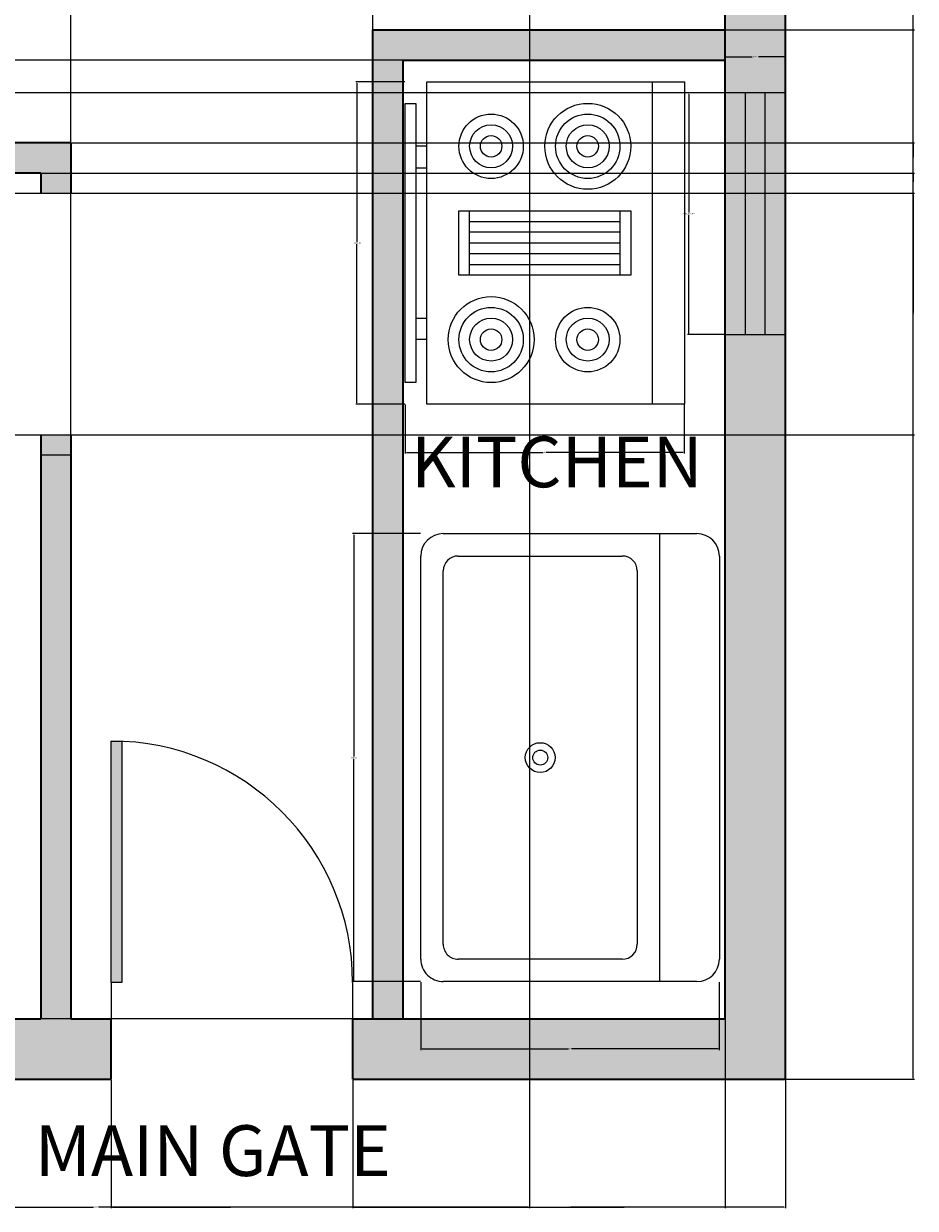
# Model space of a CAD drawing. Units: inches. Extents: x 857 to 1111, y 424 to 822.
# Tile 2 of 9: x 979 to 1111, y 424 to 600. Entities that reach past the tile are written whole.
import ezdxf

# ---------------------------------------------------------------- set-up
doc = ezdxf.new("R2010")
doc.units = ezdxf.units.IN
for name, color, linetype, lineweight in [('A-ANNO-DIMS', 2, 'Continuous', 18), ('A-ANNO-TEXT', 7, 'Continuous', 18), ('A-AREA-IDEN', 7, 'Continuous', 25), ('A-DOOR', 3, 'Continuous', 25), ('A-DOOR-PATT', 17, 'Continuous', 13), ('A-EQPM', 8, 'Continuous', 20), ('A-FLOR-FIXT', 8, 'Continuous', 20), ('A-GLAZ', 4, 'Continuous', 18), ('A-GLAZ-PATT', 9, 'Continuous', 13), ('A-WALL', 7, 'Continuous', 35), ('A-WALL-PATT', 252, 'Continuous', 13)]:
    doc.layers.add(name, color=color, linetype=linetype, lineweight=lineweight)
doc.styles.get("Standard").update_dxf_attribs({"font": 'arial.ttf'})
doc.dimstyles.get("Standard").update_dxf_attribs({"dimtxt": 0.18, "dimasz": 0.18, "dimexe": 0.18, "dimexo": 0.0625, "dimgap": 0.09, "dimtad": 0, "dimtih": 1, "dimtoh": 1, "dimdec": 4, "dimzin": 0, "dimdsep": 46, "dimtxsty": 'Standard', "dimcen": 0.09, "dimadec": 0, "dimazin": 0, "dimtfac": 1, "dimtdec": 4, "dimtofl": 0, "dimtmove": 0, "dimatfit": 3, "dimfxl": 1, "dimtolj": 1, "dimtzin": 0, "dimarcsym": 0})

# ---------------------------------------------------------------- blocks, each defined once
blk = doc.blocks.new('*U2')
for p, q in [((0, 0), (0, -6)), ((40, 0), (40, -6))]:
    blk.add_line(p, q)
blk.add_lwpolyline([(0, 0), (0, 40), (1.75, 40), (1.75, 0)], close=True)
blk.add_arc((0, 0), 40, 0, 90)
blk = doc.blocks.new('Range-Oven - 30 in top')
for p, q in [((0, -3), (30, -3)), ((12, -6), (18, -6)), ((13, -20), (13, -6)), ((14, -6), (14, -20)), ((15, -20), (15, -6)), ((16, -6), (16, -20)), ((17, -20), (17, -6)), ((18, -20), (12, -20)), ((6, -24), (6, -25)), ((8, -25), (8, -24)), ((22, -25), (22, -24)), ((24, -24), (24, -25))]:
    blk.add_line(p, q)
for points in [[(0, -24), (0, 0), (30, 0), (30, -24)], [(12, -21), (12, -5), (18, -5), (18, -21)], [(2, -26), (2, -25), (28, -25), (28, -26)]]:
    blk.add_lwpolyline(points, close=True)
for centre, radius in [((6, -9), 4), ((6, -9), 3), ((24, -9), 3), ((6, -9), 2), ((24, -9), 2), ((6, -9), 1), ((24, -9), 1), ((24, -18), 4), ((6, -18), 3), ((24, -18), 3), ((6, -18), 2), ((24, -18), 2), ((6, -18), 1), ((24, -18), 1)]:
    blk.add_circle(centre, radius)
blk = doc.blocks.new('Sink-single - 30 in top')
blk.add_line((-15, -3.999996), (15, -3.999996))
for points in [[(-13.5, 0), (13.5, 0)], [(-15, -18.499996), (-15, -1.5)], [(15, -1.5), (15, -18.499996)], [(-12.5, -5.499996), (12.5, -5.499996)], [(-13.5, -17.499996), (-13.5, -6.499996)], [(13.5, -6.499996), (13.5, -17.499996)], [(12.5, -18.499996), (-12.5, -18.499996)], [(13.5, -19.999996), (-13.5, -19.999996)]]:
    blk.add_lwpolyline(points)
for radius in [1, 0.5]:
    blk.add_circle((0, -11.999996), radius)
for centre, radius, start, end in [((-13.5, -1.5), 1.5, 90, 180), ((13.5, -1.5), 1.5, 0, 90), ((-12.5, -6.499996), 1, 90, 180), ((12.5, -6.499996), 1, 0, 90), ((-12.5, -17.499996), 1, 180, 270), ((12.5, -17.499996), 1, 270, 0), ((-13.5, -18.499996), 1.5, 180, 270), ((13.5, -18.499996), 1.5, 270, 0)]:
    blk.add_arc(centre, radius, start, end)
blk = doc.blocks.new('*U16')
for p, q in [((0, 0), (0, -6)), ((-40, 0), (-40, -6))]:
    blk.add_line(p, q)
blk.add_lwpolyline([(0, 0), (0, 40), (-1.75, 40), (-1.75, 0)], close=True)
blk.add_arc((0, 0), 40, 90, 180)
blk = doc.blocks.new('WIN-36IN-9IN-WALL')
for p, q in [((3, 36), (3, 0)), ((6, 0), (6, 36))]:
    blk.add_line(p, q)
blk.add_lwpolyline([(0, 36), (0, 0), (9, 0), (9, 36)], close=True)
blk = doc.blocks.new('*D20')
at = {"layer": 'A-ANNO-DIMS', "color": 0, "lineweight": -2, "transparency": 16777216}
for p, q in [((1083.07, 589.8), (1077.56, 589.8)), ((1077.74, 589.62), (1077.74, 571.99)), ((1077.74, 553.98), (1077.74, 571.62)), ((1083.07, 553.8), (1077.56, 553.8))]:
    blk.add_line(p, q, dxfattribs=at)
at = {"layer": 'A-ANNO-DIMS', "color": 0, "transparency": 16777216}
for points in [[(1077.71, 589.62), (1077.77, 589.62), (1077.74, 589.8)], [(1077.71, 553.98), (1077.77, 553.98), (1077.74, 553.8)]]:
    blk.add_solid(points, dxfattribs=at)
at = {"layer": 'Defpoints', "color": 0, "transparency": 16777216}
for p in [(1077.74, 589.8), (1083.14, 589.8), (1083.14, 553.8)]:
    blk.add_point(p, dxfattribs=at)
at = {"layer": 'A-ANNO-DIMS', "color": 0, "transparency": 16777216, "insert": (1077.74, 571.8), "char_height": 0.18, "attachment_point": 5}
blk.add_mtext('\\A1;WINDOW 36 TYP.', dxfattribs=at)
blk = doc.blocks.new('*D21')
at = {"layer": 'A-ANNO-DIMS', "color": 0, "lineweight": -2, "transparency": 16777216}
for p, q in [((1083.14, 589.87), (1083.14, 595.38)), ((1083.32, 595.2), (1087.18, 595.2)), ((1091.96, 595.2), (1088.1, 595.2)), ((1092.14, 589.87), (1092.14, 595.38))]:
    blk.add_line(p, q, dxfattribs=at)
at = {"layer": 'A-ANNO-DIMS', "color": 0, "transparency": 16777216}
for points in [[(1083.32, 595.23), (1083.32, 595.17), (1083.14, 595.2)], [(1091.96, 595.23), (1091.96, 595.17), (1092.14, 595.2)]]:
    blk.add_solid(points, dxfattribs=at)
at = {"layer": 'Defpoints', "color": 0, "transparency": 16777216}
for p in [(1092.14, 595.2), (1083.14, 589.8), (1092.14, 589.8)]:
    blk.add_point(p, dxfattribs=at)
at = {"layer": 'A-ANNO-DIMS', "color": 0, "transparency": 16777216, "insert": (1087.64, 595.2), "char_height": 0.18, "attachment_point": 5}
blk.add_mtext('\\A1;9 TYP.', dxfattribs=at)
blk = doc.blocks.new('*D38')
at = {"layer": 'A-ANNO-DIMS', "color": 0, "lineweight": -2, "transparency": 16777216}
for p, q in [((1035.4, 591.45), (1028.08, 591.45)), ((1028.26, 591.27), (1028.26, 567.63)), ((1028.26, 543.63), (1028.26, 567.26)), ((1035.4, 543.45), (1028.08, 543.45))]:
    blk.add_line(p, q, dxfattribs=at)
at = {"layer": 'A-ANNO-DIMS', "color": 0, "transparency": 16777216}
for points in [[(1028.23, 591.27), (1028.29, 591.27), (1028.26, 591.45)], [(1028.23, 543.63), (1028.29, 543.63), (1028.26, 543.45)]]:
    blk.add_solid(points, dxfattribs=at)
at = {"layer": 'Defpoints', "color": 0, "transparency": 16777216}
for p in [(1035.46, 591.45), (1028.26, 543.45), (1035.46, 543.45)]:
    blk.add_point(p, dxfattribs=at)
at = {"layer": 'A-ANNO-DIMS', "color": 0, "transparency": 16777216, "insert": (1028.26, 567.45), "char_height": 0.18, "attachment_point": 5}
blk.add_mtext('\\A1;RANGE 48', dxfattribs=at)
blk = doc.blocks.new('*D39')
at = {"layer": 'A-ANNO-DIMS', "color": 0, "lineweight": -2, "transparency": 16777216}
for p, q in [((1035.46, 543.38), (1035.46, 536.07)), ((1077.06, 543.38), (1077.06, 536.07)), ((1035.64, 536.25), (1056.04, 536.25)), ((1076.88, 536.25), (1056.49, 536.25))]:
    blk.add_line(p, q, dxfattribs=at)
at = {"layer": 'A-ANNO-DIMS', "color": 0, "transparency": 16777216}
for points in [[(1035.64, 536.28), (1035.64, 536.22), (1035.46, 536.25)], [(1076.88, 536.28), (1076.88, 536.22), (1077.06, 536.25)]]:
    blk.add_solid(points, dxfattribs=at)
at = {"layer": 'Defpoints', "color": 0, "transparency": 16777216}
for p in [(1035.46, 543.45), (1077.06, 543.45), (1077.06, 536.25)]:
    blk.add_point(p, dxfattribs=at)
at = {"layer": 'A-ANNO-DIMS', "color": 0, "transparency": 16777216, "insert": (1056.26, 536.25), "char_height": 0.18, "attachment_point": 5}
blk.add_mtext('\\A1;42', dxfattribs=at)
blk = doc.blocks.new('*D40')
at = {"layer": 'A-ANNO-DIMS', "color": 0, "lineweight": -2, "transparency": 16777216}
for p, q in [((1037.72, 524.14), (1027.6, 524.14)), ((1027.78, 523.96), (1027.78, 490.96)), ((1027.78, 457.58), (1027.78, 490.59)), ((1037.72, 457.4), (1027.6, 457.4))]:
    blk.add_line(p, q, dxfattribs=at)
at = {"layer": 'A-ANNO-DIMS', "color": 0, "transparency": 16777216}
for points in [[(1027.75, 523.96), (1027.81, 523.96), (1027.78, 524.14)], [(1027.75, 457.58), (1027.81, 457.58), (1027.78, 457.4)]]:
    blk.add_solid(points, dxfattribs=at)
at = {"layer": 'Defpoints', "color": 0, "transparency": 16777216}
for p in [(1037.79, 524.14), (1027.78, 457.4), (1037.79, 457.4)]:
    blk.add_point(p, dxfattribs=at)
at = {"layer": 'A-ANNO-DIMS', "color": 0, "transparency": 16777216, "insert": (1027.78, 490.77), "char_height": 0.18, "attachment_point": 5}
blk.add_mtext('\\A1;SINK 67', dxfattribs=at)
blk = doc.blocks.new('*D41')
at = {"layer": 'A-ANNO-DIMS', "color": 0, "lineweight": -2, "transparency": 16777216}
for p, q in [((1037.79, 457.34), (1037.79, 447.21)), ((1082.28, 457.34), (1082.28, 447.21)), ((1037.97, 447.39), (1059.81, 447.39)), ((1082.1, 447.39), (1060.26, 447.39))]:
    blk.add_line(p, q, dxfattribs=at)
at = {"layer": 'A-ANNO-DIMS', "color": 0, "transparency": 16777216}
for points in [[(1037.97, 447.42), (1037.97, 447.36), (1037.79, 447.39)], [(1082.1, 447.42), (1082.1, 447.36), (1082.28, 447.39)]]:
    blk.add_solid(points, dxfattribs=at)
at = {"layer": 'Defpoints', "color": 0, "transparency": 16777216}
for p in [(1037.79, 457.4), (1082.28, 457.4), (1082.28, 447.39)]:
    blk.add_point(p, dxfattribs=at)
at = {"layer": 'A-ANNO-DIMS', "color": 0, "transparency": 16777216, "insert": (1060.03, 447.39), "char_height": 0.18, "attachment_point": 5}
blk.add_mtext('\\A1;44', dxfattribs=at)
blk = doc.blocks.new('*D45')
at = {"layer": 'A-ANNO-DIMS', "color": 0, "lineweight": -2, "transparency": 16777216}
for p, q in [((1092.2, 802.86), (1111.37, 802.86)), ((1111.19, 802.68), (1111.19, 623.04)), ((1111.19, 443.04), (1111.19, 622.67)), ((1092.2, 442.86), (1111.37, 442.86))]:
    blk.add_line(p, q, dxfattribs=at)
at = {"layer": 'A-ANNO-DIMS', "color": 0, "transparency": 16777216}
for points in [[(1111.16, 802.68), (1111.22, 802.68), (1111.19, 802.86)], [(1111.16, 443.04), (1111.22, 443.04), (1111.19, 442.86)]]:
    blk.add_solid(points, dxfattribs=at)
at = {"layer": 'Defpoints', "color": 0, "transparency": 16777216}
for p in [(1092.14, 802.86), (1111.19, 802.86), (1092.14, 442.86)]:
    blk.add_point(p, dxfattribs=at)
at = {"layer": 'A-ANNO-DIMS', "color": 0, "transparency": 16777216, "insert": (1111.19, 622.86), "char_height": 0.18, "attachment_point": 5}
blk.add_mtext('\\A1;360', dxfattribs=at)
blk = doc.blocks.new('*D46')
at = {"layer": 'A-ANNO-DIMS', "color": 0, "lineweight": -2, "transparency": 16777216}
for p, q in [((991.64, 442.79), (991.64, 423.63)), ((1027.64, 442.79), (1027.64, 423.63)), ((991.82, 423.81), (1009.42, 423.81)), ((1027.46, 423.81), (1009.86, 423.81))]:
    blk.add_line(p, q, dxfattribs=at)
at = {"layer": 'A-ANNO-DIMS', "color": 0, "transparency": 16777216}
for points in [[(991.82, 423.84), (991.82, 423.78), (991.64, 423.81)], [(1027.46, 423.84), (1027.46, 423.78), (1027.64, 423.81)]]:
    blk.add_solid(points, dxfattribs=at)
at = {"layer": 'Defpoints', "color": 0, "transparency": 16777216}
for p in [(991.64, 442.86), (1027.64, 442.86), (1027.64, 423.81)]:
    blk.add_point(p, dxfattribs=at)
at = {"layer": 'A-ANNO-DIMS', "color": 0, "transparency": 16777216, "insert": (1009.64, 423.81), "char_height": 0.18, "attachment_point": 5}
blk.add_mtext('\\A1;36', dxfattribs=at)
blk = doc.blocks.new('*D47')
at = {"layer": 'A-ANNO-DIMS', "color": 0, "lineweight": -2, "transparency": 16777216}
for p, q in [((1027.64, 442.79), (1027.64, 423.63)), ((1092.14, 442.79), (1092.14, 423.63)), ((1027.82, 423.81), (1059.56, 423.81)), ((1091.96, 423.81), (1060.21, 423.81))]:
    blk.add_line(p, q, dxfattribs=at)
at = {"layer": 'A-ANNO-DIMS', "color": 0, "transparency": 16777216}
for points in [[(1027.82, 423.84), (1027.82, 423.78), (1027.64, 423.81)], [(1091.96, 423.84), (1091.96, 423.78), (1092.14, 423.81)]]:
    blk.add_solid(points, dxfattribs=at)
at = {"layer": 'Defpoints', "color": 0, "transparency": 16777216}
for p in [(1027.64, 442.86), (1092.14, 442.86), (1092.14, 423.81)]:
    blk.add_point(p, dxfattribs=at)
at = {"layer": 'A-ANNO-DIMS', "color": 0, "transparency": 16777216, "insert": (1059.89, 423.81), "char_height": 0.18, "attachment_point": 5}
blk.add_mtext('\\A1;64.5', dxfattribs=at)
blk = doc.blocks.new('*D48')
at = {"layer": 'A-ANNO-DIMS', "color": 0, "lineweight": -2, "transparency": 16777216}
for p, q in [((885.14, 582.42), (885.14, 822.09)), ((885.32, 821.91), (935, 821.91)), ((985.46, 821.91), (935.77, 821.91)), ((985.64, 582.42), (985.64, 822.09))]:
    blk.add_line(p, q, dxfattribs=at)
at = {"layer": 'A-ANNO-DIMS', "color": 0, "transparency": 16777216}
for points in [[(885.32, 821.94), (885.32, 821.88), (885.14, 821.91)], [(985.46, 821.94), (985.46, 821.88), (985.64, 821.91)]]:
    blk.add_solid(points, dxfattribs=at)
at = {"layer": 'Defpoints', "color": 0, "transparency": 16777216}
for p in [(985.64, 821.91), (885.14, 582.36), (985.64, 582.36)]:
    blk.add_point(p, dxfattribs=at)
at = {"layer": 'A-ANNO-DIMS', "color": 0, "transparency": 16777216, "insert": (935.39, 821.91), "char_height": 0.18, "attachment_point": 5}
blk.add_mtext('\\A1;100.5', dxfattribs=at)
blk = doc.blocks.new('*D49')
at = {"layer": 'A-ANNO-DIMS', "color": 0, "lineweight": -2, "transparency": 16777216}
for p, q in [((985.64, 451.92), (985.64, 822.09)), ((985.82, 821.91), (1007.91, 821.91)), ((1030.46, 821.91), (1008.36, 821.91)), ((1030.64, 451.92), (1030.64, 822.09))]:
    blk.add_line(p, q, dxfattribs=at)
at = {"layer": 'A-ANNO-DIMS', "color": 0, "transparency": 16777216}
for points in [[(985.82, 821.94), (985.82, 821.88), (985.64, 821.91)], [(1030.46, 821.94), (1030.46, 821.88), (1030.64, 821.91)]]:
    blk.add_solid(points, dxfattribs=at)
at = {"layer": 'Defpoints', "color": 0, "transparency": 16777216}
for p in [(1030.64, 821.91), (985.64, 451.86), (1030.64, 451.86)]:
    blk.add_point(p, dxfattribs=at)
at = {"layer": 'A-ANNO-DIMS', "color": 0, "transparency": 16777216, "insert": (1008.14, 821.91), "char_height": 0.18, "attachment_point": 5}
blk.add_mtext('\\A1;45', dxfattribs=at)
blk = doc.blocks.new('*D50')
at = {"layer": 'A-ANNO-DIMS', "color": 0, "lineweight": -2, "transparency": 16777216}
for p, q in [((981.2, 577.86), (1111.37, 577.86)), ((1111.19, 577.68), (1111.19, 576.54)), ((1111.19, 575.04), (1111.19, 576.17)), ((981.2, 574.86), (1111.37, 574.86))]:
    blk.add_line(p, q, dxfattribs=at)
at = {"layer": 'A-ANNO-DIMS', "color": 0, "transparency": 16777216}
for points in [[(1111.16, 577.68), (1111.22, 577.68), (1111.19, 577.86)], [(1111.16, 575.04), (1111.22, 575.04), (1111.19, 574.86)]]:
    blk.add_solid(points, dxfattribs=at)
at = {"layer": 'Defpoints', "color": 0, "transparency": 16777216}
for p in [(981.14, 577.86), (1111.19, 577.86), (981.14, 574.86)]:
    blk.add_point(p, dxfattribs=at)
at = {"layer": 'A-ANNO-DIMS', "color": 0, "transparency": 16777216, "insert": (1111.19, 576.36), "char_height": 0.18, "attachment_point": 5}
blk.add_mtext('\\A1;3', dxfattribs=at)
blk = doc.blocks.new('*D51')
at = {"layer": 'A-ANNO-DIMS', "color": 0, "lineweight": -2, "transparency": 16777216}
for p, q in [((985.7, 574.86), (1111.37, 574.86)), ((1111.19, 574.68), (1111.19, 557.04)), ((1111.19, 539.04), (1111.19, 556.67)), ((985.7, 538.86), (1111.37, 538.86))]:
    blk.add_line(p, q, dxfattribs=at)
at = {"layer": 'A-ANNO-DIMS', "color": 0, "transparency": 16777216}
for points in [[(1111.16, 574.68), (1111.22, 574.68), (1111.19, 574.86)], [(1111.16, 539.04), (1111.22, 539.04), (1111.19, 538.86)]]:
    blk.add_solid(points, dxfattribs=at)
at = {"layer": 'Defpoints', "color": 0, "transparency": 16777216}
for p in [(985.64, 574.86), (1111.19, 574.86), (985.64, 538.86)]:
    blk.add_point(p, dxfattribs=at)
at = {"layer": 'A-ANNO-DIMS', "color": 0, "transparency": 16777216, "insert": (1111.19, 556.86), "char_height": 0.18, "attachment_point": 5}
blk.add_mtext('\\A1;36', dxfattribs=at)
blk = doc.blocks.new('*D52')
at = {"layer": 'A-ANNO-DIMS', "color": 0, "lineweight": -2, "transparency": 16777216}
for p, q in [((985.7, 582.36), (1111.37, 582.36)), ((1111.19, 582.18), (1111.19, 580.29)), ((1111.19, 578.04), (1111.19, 579.93)), ((981.2, 577.86), (1111.37, 577.86))]:
    blk.add_line(p, q, dxfattribs=at)
at = {"layer": 'A-ANNO-DIMS', "color": 0, "transparency": 16777216}
for points in [[(1111.16, 582.18), (1111.22, 582.18), (1111.19, 582.36)], [(1111.16, 578.04), (1111.22, 578.04), (1111.19, 577.86)]]:
    blk.add_solid(points, dxfattribs=at)
at = {"layer": 'Defpoints', "color": 0, "transparency": 16777216}
for p in [(985.64, 582.36), (1111.19, 582.36), (981.14, 577.86)]:
    blk.add_point(p, dxfattribs=at)
at = {"layer": 'A-ANNO-DIMS', "color": 0, "transparency": 16777216, "insert": (1111.19, 580.11), "char_height": 0.18, "attachment_point": 5}
blk.add_mtext('\\A1;4.5', dxfattribs=at)
blk = doc.blocks.new('*D53')
at = {"layer": 'A-ANNO-DIMS', "color": 0, "lineweight": -2, "transparency": 16777216}
for p, q in [((1035.07, 594.69), (856.91, 594.69)), ((857.09, 594.51), (857.09, 523.46)), ((857.09, 452.04), (857.09, 523.09)), ((1035.07, 451.86), (856.91, 451.86))]:
    blk.add_line(p, q, dxfattribs=at)
at = {"layer": 'A-ANNO-DIMS', "color": 0, "transparency": 16777216}
for points in [[(857.06, 594.51), (857.12, 594.51), (857.09, 594.69)], [(857.06, 452.04), (857.12, 452.04), (857.09, 451.86)]]:
    blk.add_solid(points, dxfattribs=at)
at = {"layer": 'Defpoints', "color": 0, "transparency": 16777216}
for p in [(857.09, 594.69), (1035.14, 594.69), (1035.14, 451.86)]:
    blk.add_point(p, dxfattribs=at)
at = {"layer": 'A-ANNO-DIMS', "color": 0, "transparency": 16777216, "insert": (857.09, 523.28), "char_height": 0.18, "attachment_point": 5}
blk.add_mtext('\\A1;142.84', dxfattribs=at)
blk = doc.blocks.new('*D55')
at = {"layer": 'A-ANNO-DIMS', "color": 0, "lineweight": -2, "transparency": 16777216}
for p, q in [((1053.97, 717.29), (1053.97, 423.63)), ((1083.14, 717.29), (1083.14, 423.63)), ((1054.15, 423.81), (1068.09, 423.81)), ((1082.96, 423.81), (1069.02, 423.81))]:
    blk.add_line(p, q, dxfattribs=at)
at = {"layer": 'A-ANNO-DIMS', "color": 0, "transparency": 16777216}
for points in [[(1054.15, 423.84), (1054.15, 423.78), (1053.97, 423.81)], [(1082.96, 423.84), (1082.96, 423.78), (1083.14, 423.81)]]:
    blk.add_solid(points, dxfattribs=at)
at = {"layer": 'Defpoints', "color": 0, "transparency": 16777216}
for p in [(1053.97, 717.36), (1083.14, 717.36), (1083.14, 423.81)]:
    blk.add_point(p, dxfattribs=at)
at = {"layer": 'A-ANNO-DIMS', "color": 0, "transparency": 16777216, "insert": (1068.55, 423.81), "char_height": 0.18, "attachment_point": 5}
blk.add_mtext('\\A1;29.165', dxfattribs=at)
blk = doc.blocks.new('*D56')
at = {"layer": 'A-ANNO-DIMS', "color": 0, "lineweight": -2, "transparency": 16777216}
for p, q in [((924.77, 717.29), (924.77, 423.63)), ((1053.97, 717.29), (1053.97, 423.63)), ((924.95, 423.81), (988.99, 423.81)), ((1053.79, 423.81), (989.75, 423.81))]:
    blk.add_line(p, q, dxfattribs=at)
at = {"layer": 'A-ANNO-DIMS', "color": 0, "transparency": 16777216}
for points in [[(924.95, 423.84), (924.95, 423.78), (924.77, 423.81)], [(1053.79, 423.84), (1053.79, 423.78), (1053.97, 423.81)]]:
    blk.add_solid(points, dxfattribs=at)
at = {"layer": 'Defpoints', "color": 0, "transparency": 16777216}
for p in [(924.77, 717.36), (1053.97, 717.36), (1053.97, 423.81)]:
    blk.add_point(p, dxfattribs=at)
at = {"layer": 'A-ANNO-DIMS', "color": 0, "transparency": 16777216, "insert": (989.37, 423.81), "char_height": 0.18, "attachment_point": 5}
blk.add_mtext('\\A1;129.2', dxfattribs=at)
blk = doc.blocks.new('*D60')
at = {"layer": 'A-ANNO-DIMS', "color": 0, "lineweight": -2, "transparency": 16777216}
for p, q in [((1083.07, 594.69), (856.91, 594.69)), ((857.09, 594.51), (857.09, 592.43)), ((857.09, 589.98), (857.09, 592.07)), ((1083.07, 589.8), (856.91, 589.8))]:
    blk.add_line(p, q, dxfattribs=at)
at = {"layer": 'A-ANNO-DIMS', "color": 0, "transparency": 16777216}
for points in [[(857.06, 594.51), (857.12, 594.51), (857.09, 594.69)], [(857.06, 589.98), (857.12, 589.98), (857.09, 589.8)]]:
    blk.add_solid(points, dxfattribs=at)
at = {"layer": 'Defpoints', "color": 0, "transparency": 16777216}
for p in [(857.09, 594.69), (1083.14, 594.69), (1083.14, 589.8)]:
    blk.add_point(p, dxfattribs=at)
at = {"layer": 'A-ANNO-DIMS', "color": 0, "transparency": 16777216, "insert": (857.09, 592.25), "char_height": 0.18, "attachment_point": 5}
blk.add_mtext('\\A1;4.891', dxfattribs=at)
blk = doc.blocks.new('*D61')
at = {"layer": 'A-ANNO-DIMS', "color": 0, "lineweight": -2, "transparency": 16777216}
for p, q in [((1083.2, 670.61), (1111.37, 670.61)), ((1111.19, 670.43), (1111.19, 635.08)), ((1111.19, 599.37), (1111.19, 634.72)), ((1083.2, 599.19), (1111.37, 599.19))]:
    blk.add_line(p, q, dxfattribs=at)
at = {"layer": 'A-ANNO-DIMS', "color": 0, "transparency": 16777216}
for points in [[(1111.16, 670.43), (1111.22, 670.43), (1111.19, 670.61)], [(1111.16, 599.37), (1111.22, 599.37), (1111.19, 599.19)]]:
    blk.add_solid(points, dxfattribs=at)
at = {"layer": 'Defpoints', "color": 0, "transparency": 16777216}
for p in [(1083.14, 670.61), (1111.19, 670.61), (1083.14, 599.19)]:
    blk.add_point(p, dxfattribs=at)
at = {"layer": 'A-ANNO-DIMS', "color": 0, "transparency": 16777216, "insert": (1111.19, 634.9), "char_height": 0.18, "attachment_point": 5}
blk.add_mtext('\\A1;71.41', dxfattribs=at)

msp = doc.modelspace()

# ---------------------------------------------------------------- hatches: boundary and pattern name
at = {"layer": 'A-DOOR-PATT'}
h = msp.add_hatch(color=256, dxfattribs=at)
h.dxf.hatch_style = 1
h.paths.add_polyline_path([(975.7391, 574.8417), (939.754, 574.8417, 0.01094143), (939.7885, 573.2674), (975.7391, 573.2674)])
h.paths.add_polyline_path([(985.6369, 577.8567), (981.1369, 577.8567), (981.1369, 574.8567), (985.6369, 574.8567)])
h.paths.add_polyline_path([(985.6369, 538.8567), (981.1369, 538.8567), (981.1369, 535.8567), (985.6369, 535.8567)])
h.paths.add_polyline_path([(993.2112, 493.205, 0.01094143), (991.6369, 493.2395), (991.6369, 457.2544), (993.2112, 457.2544)])
at = {"layer": 'A-GLAZ-PATT'}
h = msp.add_hatch(color=256, dxfattribs=at)
h.dxf.hatch_style = 1
h.set_gradient(color1=(0, 0, 255), color2=(255, 255, 0), name='INVCURVED')
h.paths.add_polyline_path([(1092.1369, 589.8025), (1089.1369, 589.8025), (1089.1369, 553.8025), (1092.1369, 553.8025)])
h.paths.add_polyline_path([(1089.1369, 589.8025), (1086.1369, 589.8025), (1086.1369, 553.8025), (1089.1369, 553.8025)])
h.paths.add_polyline_path([(1086.1369, 589.8025), (1083.1369, 589.8025), (1083.1369, 553.8025), (1086.1369, 553.8025)])
at = {"layer": 'A-WALL-PATT'}
h = msp.add_hatch(color=256, dxfattribs=at)
h.dxf.hatch_style = 1
h.paths.add_polyline_path([(924.7696, 721.8567), (885.1369, 721.8567), (885.1369, 793.8567), (1083.1369, 793.8567), (1083.1369, 721.8567), (1053.9717, 721.8567), (1053.9717, 717.3567), (1083.1369, 717.3567), (1083.1369, 706.6069), (1092.1369, 706.6069), (1092.1369, 802.8567), (876.1369, 802.8567), (876.1369, 664.6868), (885.1369, 664.6868), (885.1369, 717.3567), (924.7696, 717.3567)])
h.paths.add_polyline_path([(985.6369, 582.3567), (885.1369, 582.3567), (885.1369, 585.1154), (885.1369, 628.6868), (876.1369, 628.6868), (876.1369, 529.0363), (885.1369, 529.0363), (885.1369, 577.8567), (981.1369, 577.8567), (985.6369, 577.8567)])
h.paths.add_polyline_path([(885.1369, 493.0363), (876.1369, 493.0363), (876.1369, 442.8567), (991.6369, 442.8567), (991.6369, 451.8567), (985.6369, 451.8567), (985.6369, 535.8567), (981.1369, 535.8567), (981.1369, 451.8567), (885.1369, 451.8567)])
h.paths.add_polyline_path([(1092.1369, 553.8025), (1083.1369, 553.8025), (1083.1369, 451.8567), (1030.6369, 451.8567), (1027.6369, 451.8567), (1027.6369, 442.8567), (1092.1369, 442.8567)])
h.paths.add_polyline_path([(1092.1369, 670.6069), (1083.1369, 670.6069), (1083.1369, 662.5384, -0.02676862), (1083.1369, 657.4501), (1083.1369, 589.8025), (1092.1369, 589.8025)])
h = msp.add_hatch(color=256, dxfattribs=at)
h.dxf.hatch_style = 1
h.paths.add_polyline_path([(1035.1369, 594.6935), (1083.1369, 594.6935), (1083.1369, 599.1935), (1030.6369, 599.1935), (1030.6369, 451.8567), (1035.1369, 451.8567)])

# ---------------------------------------------------------------- linework, layer by layer
at = {"layer": 'A-DOOR'}
for p, q in [((981.1369, 577.8567), (985.6369, 577.8567)), ((981.1369, 574.8567), (985.6369, 574.8567)), ((981.1369, 538.8567), (985.6369, 538.8567)), ((981.1369, 535.8567), (985.6369, 535.8567))]:
    msp.add_line(p, q, dxfattribs=at)
at = {"layer": 'A-WALL'}
for p, q in [((1083.1369, 451.8567), (1083.1369, 717.3567)), ((1030.6369, 599.1935), (1083.1369, 599.1935)), ((1030.6369, 451.8567), (1030.6369, 599.1935)), ((1035.1369, 451.8567), (1035.1369, 594.6935)), ((1035.1369, 594.6935), (1083.1369, 594.6935)), ((985.6369, 582.3567), (885.1369, 582.3567)), ((985.6369, 582.3567), (985.6369, 574.8567)), ((981.1369, 577.8567), (885.1369, 577.8567)), ((981.1369, 577.8567), (981.1369, 574.8567)), ((981.1369, 538.8567), (981.1369, 451.8567)), ((985.6369, 538.8567), (985.6369, 451.8567)), ((885.1369, 451.8567), (981.1369, 451.8567)), ((985.6369, 451.8567), (991.6369, 451.8567)), ((991.6369, 442.8567), (991.6369, 451.8567)), ((1027.6369, 442.8567), (1027.6369, 451.8567)), ((1027.6369, 451.8567), (1030.6369, 451.8567)), ((1030.6369, 451.8567), (1083.1369, 451.8567))]:
    msp.add_line(p, q, dxfattribs=at)
msp.add_lwpolyline([(1027.6369, 442.8567), (1092.1369, 442.8567), (1092.1369, 802.8567), (876.1369, 802.8567), (876.1369, 442.8567), (991.6369, 442.8567)], dxfattribs=at)

# ---------------------------------------------------------------- block references
at = {"layer": 'A-DOOR', "xscale": 0.8996270808511326, "yscale": 0.8996270808511326, "zscale": 0.8996270808511326, "rotation": 90}
msp.add_blockref('*U16', (975.7391, 574.8417), dxfattribs=at)
at = {"layer": 'A-DOOR', "xscale": 0.8996270808511326, "yscale": 0.8996270808511326, "zscale": 0.8996270808511326}
msp.add_blockref('*U2', (991.6369, 457.2544), dxfattribs=at)
at = {"layer": 'A-EQPM', "xscale": 1.6, "yscale": 1.6, "zscale": 1.6, "rotation": 270}
msp.add_blockref('Range-Oven - 30 in top', (1077.0645, 591.4461), dxfattribs=at)
at = {"layer": 'A-FLOR-FIXT', "xscale": 2.224697682963642, "yscale": 2.224697682963642, "zscale": 2.224697682963642, "rotation": 270}
msp.add_blockref('Sink-single - 30 in top', (1082.2811, 490.7738), dxfattribs=at)
at = {"layer": 'A-GLAZ'}
msp.add_blockref('WIN-36IN-9IN-WALL', (1083.1369, 553.8025), dxfattribs=at)

# ---------------------------------------------------------------- texts
at = {"layer": 'A-ANNO-TEXT'}
msp.add_text('MAIN GATE ', height=7.55928, dxfattribs=at).set_placement((980.2531, 428.4368))
at = {"layer": 'A-AREA-IDEN'}
msp.add_text('KITCHEN ', height=7.55928, dxfattribs=at).set_placement((1036.3194, 531.0461))

# ---------------------------------------------------------------- dimensions: what is measured, and where the dimension line sits
at = {"layer": 'A-ANNO-DIMS'}
for base, p1, p2, override, picture, middle in [((985.6369, 821.9067), (885.1369, 582.3567), (985.6369, 582.3567), {"dimdec": 1, "dimlfac": 1, "dimrnd": 0, "dimzin": 0, "dimdsep": 46, "dimlunit": 2}, '*D48', (935.3869, 821.9067)), ((1030.6369, 821.9067), (985.6369, 451.8567), (1030.6369, 451.8567), {"dimdec": 0, "dimlfac": 1, "dimrnd": 0, "dimzin": 0, "dimdsep": 46, "dimlunit": 2}, '*D49', (1008.1369, 821.9067)), ((1053.9717, 423.8067), (924.7696, 717.3567), (1053.9717, 717.3567), {"dimdec": 1, "dimlfac": 1, "dimrnd": 0, "dimzin": 0, "dimdsep": 46, "dimlunit": 2}, '*D56', (989.3707, 423.8067)), ((1083.1369, 423.8067), (1053.9717, 717.3567), (1083.1369, 717.3567), {"dimdec": 3, "dimlfac": 1, "dimrnd": 0, "dimzin": 0, "dimdsep": 46, "dimlunit": 2}, '*D55', (1068.5543, 423.8067)), ((1077.0645, 536.2461), (1035.4645, 543.4461), (1077.0645, 543.4461), {"dimdec": 0, "dimlfac": 1, "dimrnd": 0, "dimzin": 0, "dimdsep": 46, "dimlunit": 2}, '*D39', (1056.2645, 536.2461)), ((1082.2811, 447.3922), (1037.7872, 457.4034), (1082.2811, 457.4034), {"dimdec": 0, "dimlfac": 1, "dimrnd": 0, "dimzin": 0, "dimdsep": 46, "dimlunit": 2}, '*D41', (1060.0341, 447.3922)), ((1027.6369, 423.8067), (991.6369, 442.8567), (1027.6369, 442.8567), {"dimdec": 0, "dimlfac": 1, "dimrnd": 0, "dimzin": 0, "dimdsep": 46, "dimlunit": 2}, '*D46', (1009.6369, 423.8067)), ((1092.1369, 423.8067), (1027.6369, 442.8567), (1092.1369, 442.8567), {"dimdec": 1, "dimlfac": 1, "dimrnd": 0, "dimzin": 0, "dimdsep": 46, "dimlunit": 2}, '*D47', (1059.8869, 423.8067))]:
    dim = msp.add_linear_dim(base=base, p1=p1, p2=p2, dimstyle='Standard', override=override, dxfattribs=at)
    dim.commit()
    dim.dimension.update_dxf_attribs({"geometry": picture, "text_midpoint": middle})
for base, p1, p2, override, picture, middle in [((1111.1869, 802.8567), (1092.1369, 442.8567), (1092.1369, 802.8567), {"dimdec": 0, "dimlfac": 1, "dimrnd": 0, "dimzin": 0, "dimdsep": 46, "dimlunit": 2}, '*D45', (1111.1869, 622.8567)), ((1111.1869, 670.6069), (1083.1369, 599.1935), (1083.1369, 670.6069), {"dimdec": 2, "dimlfac": 1, "dimrnd": 0, "dimzin": 0, "dimdsep": 46, "dimlunit": 2}, '*D61', (1111.1869, 634.9002)), ((857.0869, 594.6935), (1035.1369, 451.8567), (1035.1369, 594.6935), {"dimdec": 2, "dimlfac": 1, "dimrnd": 0, "dimzin": 0, "dimdsep": 46, "dimlunit": 2}, '*D53', (857.0869, 523.2751)), ((857.0869, 594.6935), (1083.1369, 589.8025), (1083.1369, 594.6935), {"dimdec": 3, "dimlfac": 1, "dimrnd": 0, "dimzin": 0, "dimdsep": 46, "dimlunit": 2}, '*D60', (857.0869, 592.248)), ((1111.1869, 582.3567), (981.1369, 577.8567), (985.6369, 582.3567), {"dimdec": 1, "dimlfac": 1, "dimrnd": 0, "dimzin": 0, "dimdsep": 46, "dimlunit": 2}, '*D52', (1111.1869, 580.1067)), ((1111.1869, 577.8567), (981.1369, 574.8567), (981.1369, 577.8567), {"dimdec": 0, "dimlfac": 1, "dimrnd": 0, "dimzin": 0, "dimdsep": 46, "dimlunit": 2}, '*D50', (1111.1869, 576.3567)), ((1111.1869, 574.8567), (985.6369, 538.8567), (985.6369, 574.8567), {"dimdec": 0, "dimlfac": 1, "dimrnd": 0, "dimzin": 0, "dimdsep": 46, "dimlunit": 2}, '*D51', (1111.1869, 556.8567))]:
    dim = msp.add_linear_dim(base=base, p1=p1, p2=p2, angle=90, dimstyle='Standard', override=override, dxfattribs=at)
    dim.commit()
    dim.dimension.update_dxf_attribs({"geometry": picture, "text_midpoint": middle})
dim = msp.add_linear_dim(base=(1092.1369, 595.2025), p1=(1083.1369, 589.8025), p2=(1092.1369, 589.8025), text='<> TYP.', dimstyle='Standard', override={"dimdec": 0, "dimlfac": 1, "dimrnd": 0, "dimzin": 0, "dimdsep": 46, "dimlunit": 2}, dxfattribs=at)
dim.commit()
dim.dimension.update_dxf_attribs({"geometry": '*D21', "text_midpoint": (1087.6369, 595.2025)})
for base, p1, p2, angle, text, picture, middle in [((1028.2645, 543.4461), (1035.4645, 591.4461), (1035.4645, 543.4461), 270, 'RANGE <>', '*D38', (1028.2645, 567.4461)), ((1077.7369, 589.8025), (1083.1369, 553.8025), (1083.1369, 589.8025), 90, 'WINDOW <> TYP.', '*D20', (1077.7369, 571.8025)), ((1027.776, 457.4034), (1037.7872, 524.1443), (1037.7872, 457.4034), 270, 'SINK <>', '*D40', (1027.776, 490.7738))]:
    dim = msp.add_linear_dim(base=base, p1=p1, p2=p2, angle=angle, text=text, dimstyle='Standard', override={"dimdec": 0, "dimlfac": 1, "dimrnd": 0, "dimzin": 0, "dimdsep": 46, "dimlunit": 2}, dxfattribs=at)
    dim.commit()
    dim.dimension.update_dxf_attribs({"geometry": picture, "text_midpoint": middle})

doc.saveas('drawing.dxf')
